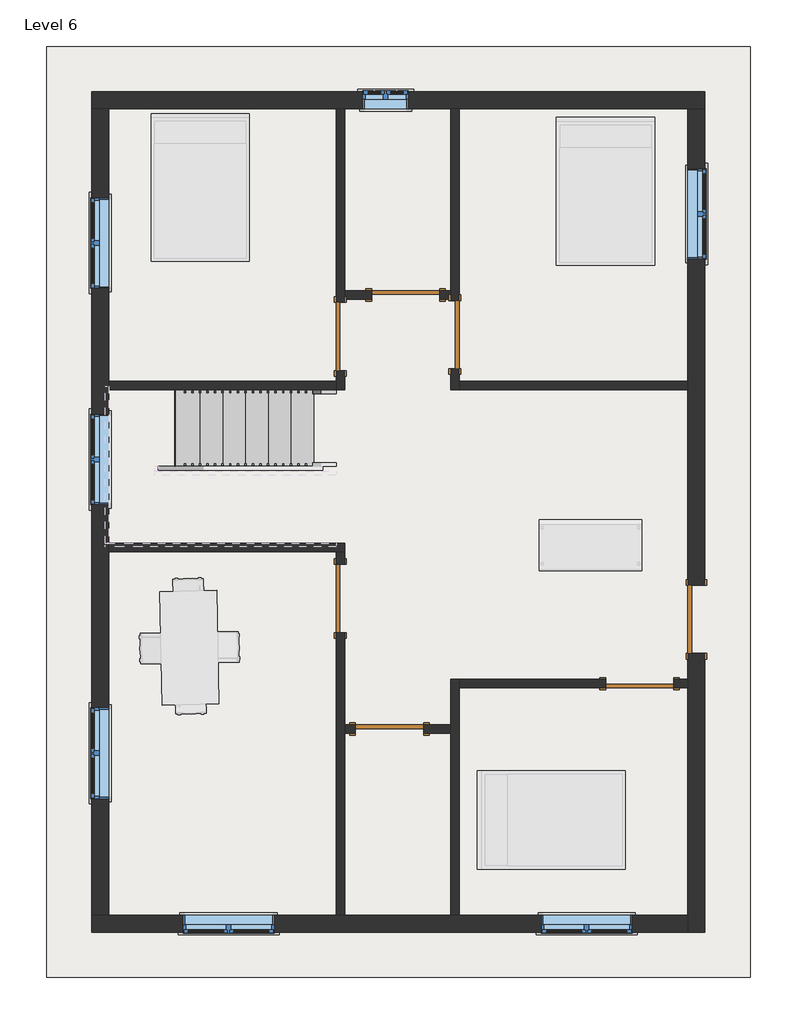
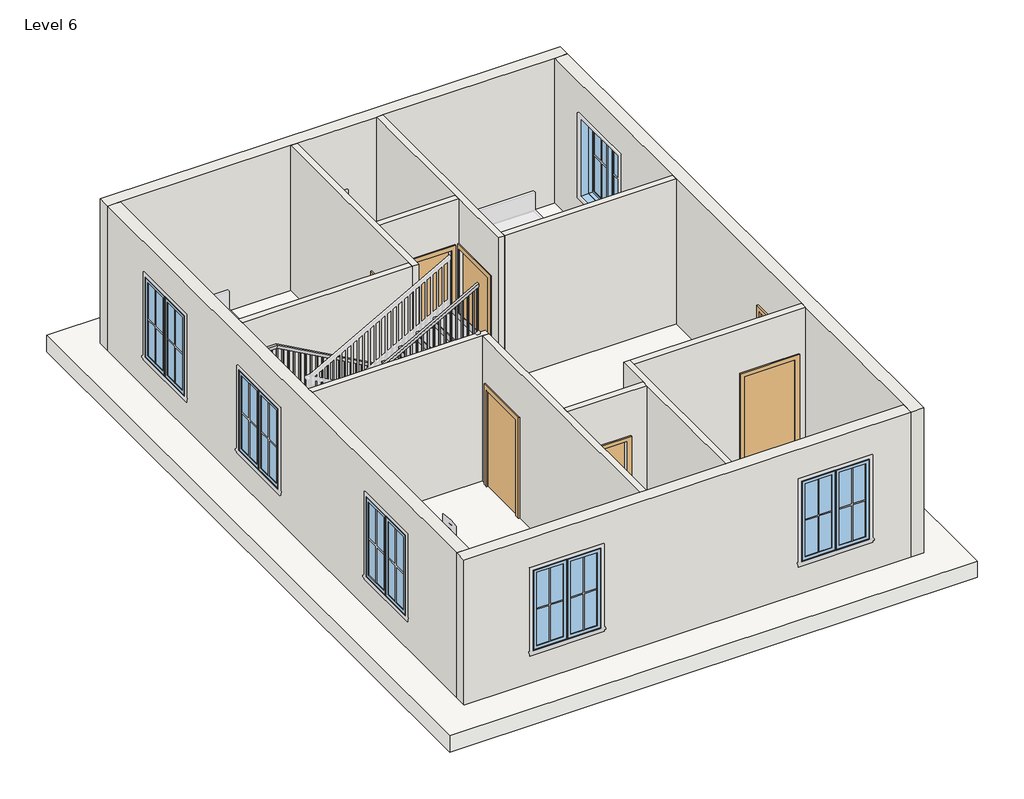
# One storey, part 1 of 2: 14 walls, 7 doors, 7 windows, 1 railing, 1 roof, 1 stair flight.
"""IFC4 building model written with IfcOpenShell, lengths in millimetres."""

from ifc_helpers import new_model, si_unit, frame, origin, place, context, project, spatial, polyline, outline, extrude, faceted_brep, transform, mapped, element, save
from components import door_e5f9f3c4, door_305aa2a5, door_a90ba1ad, stair_flight_597ccfed, window_c417fced, window_8377141f

model = new_model("IFC4")

# Units and contexts
model_context = context("Model", 3, world=origin())
ifc_project = project(units=[si_unit("LENGTHUNIT", "METRE", prefix="MILLI")], contexts=[model_context])

# Site, building, storey
site = spatial("IfcSite", under=ifc_project)
building = spatial("IfcBuilding", under=site)
storey = spatial("IfcBuildingStorey", under=building, Name="Level 6", Elevation=15240.0)

# Doors
placement = place(None, origin())
door_shape = door_e5f9f3c4(model_context)
element("IfcDoor", 1, ObjectType="Single-Flush : 36\" x 84\"", at=placement, inside=storey, context=model_context, shape_type="MappedRepresentation", body=[
    mapped(door_shape, transform((5226.05, 11245.85, 15240.0), x_axis=(1.0, 0.0, 0.0), y_axis=(0.0, 1.0, 0.0), z_axis=(0.0, 0.0, 1.0))),
])
element("IfcDoor", 2, ObjectType="Single-Flush : 36\" x 84\"", at=placement, inside=storey, context=model_context, shape_type="MappedRepresentation", body=[
    mapped(door_shape, transform((5886.45, 10712.45, 15240.0), x_axis=(0.0, -1.0, 0.0), y_axis=(1.0, 0.0, 0.0), z_axis=(0.0, 0.0, 1.0))),
])
door_2_shape = door_305aa2a5(model_context)
element("IfcDoor", 3, ObjectType="Single-Flush : 36\" x 84\"", at=placement, inside=storey, context=model_context, shape_type="MappedRepresentation", body=[
    mapped(door_2_shape, transform((4349.75, 10687.05, 15240.0), x_axis=(0.0, -1.0, 0.0), y_axis=(1.0, 0.0, 0.0), z_axis=(0.0, 0.0, 1.0))),
])
element("IfcDoor", 4, ObjectType="Single-Flush : 36\" x 84\"", at=placement, inside=storey, context=model_context, shape_type="MappedRepresentation", body=[
    mapped(door_2_shape, transform((8369.3, 6026.15, 15240.0), x_axis=(1.0, 0.0, 0.0), y_axis=(0.0, 1.0, 0.0), z_axis=(0.0, 0.0, 1.0))),
])
element("IfcDoor", 5, ObjectType="Single-Flush : 36\" x 84\"", at=placement, inside=storey, context=model_context, shape_type="MappedRepresentation", body=[
    mapped(door_2_shape, transform((5010.15, 5416.55, 15240.0), x_axis=(-1.0, 0.0, 0.0), y_axis=(0.0, -1.0, 0.0), z_axis=(0.0, 0.0, 1.0))),
])
element("IfcDoor", 6, ObjectType="Single-Flush : 36\" x 84\"", at=placement, inside=storey, context=model_context, shape_type="MappedRepresentation", body=[
    mapped(door_2_shape, transform((4349.75, 7169.15, 15240.0), x_axis=(0.0, -1.0, 0.0), y_axis=(1.0, 0.0, 0.0), z_axis=(0.0, 0.0, 1.0))),
])
door_3_shape = door_a90ba1ad(model_context)
element("IfcDoor", 7, ObjectType="Single-Flush : 36\" x 84\"", at=placement, inside=storey, context=model_context, shape_type="MappedRepresentation", body=[
    mapped(door_3_shape, transform((9131.3, 6889.75, 15240.0), x_axis=(0.0, -1.0, 0.0), y_axis=(1.0, 0.0, 0.0), z_axis=(0.0, 0.0, 1.0))),
])

# Railing
element("IfcRailing", 8, ObjectType="Handrail - Rectangular", at=placement, inside=storey, context=model_context, shape_type="SolidModel", body=[
    faceted_brep([(4295.1355783, 9918.7, 16323.7333333), (4295.1355783, 9918.7, 16265.620221), (4295.1355783, 9969.5, 16265.620221), (4295.1355783, 9969.5, 16323.7333333), (1856.7355783, 9918.7, 17678.4), (1843.5719761, 9918.7, 17627.6), (1843.5719761, 9969.5, 17627.6), (1856.7355783, 9969.5, 17678.4), (1295.4, 9918.7, 17678.4), (1295.4, 9918.7, 17627.6), (1244.6, 9969.5, 17627.6), (1244.6, 9969.5, 17678.4), (1295.4, 7962.9, 17678.4), (1295.4, 7962.9, 17627.6), (1244.6, 7912.1, 17627.6), (1244.6, 7912.1, 17678.4), (1551.9355783, 7962.9, 17678.4), (1565.0991806, 7962.9, 17627.6), (1565.0991806, 7912.1, 17627.6), (1551.9355783, 7912.1, 17678.4), (4295.1355783, 7962.9, 19202.4), (4295.1355783, 7912.1, 19202.4), (4295.1355783, 7912.1, 19144.2868876), (4295.1355783, 7962.9, 19144.2868876)], [[[0, 1, 2, 3]], [[1, 0, 4, 5]], [[2, 1, 5, 6]], [[3, 2, 6, 7]], [[0, 3, 7, 4]], [[5, 4, 8, 9]], [[6, 5, 9, 10]], [[7, 6, 10, 11]], [[4, 7, 11, 8]], [[9, 8, 12, 13]], [[10, 9, 13, 14]], [[11, 10, 14, 15]], [[8, 11, 15, 12]], [[13, 12, 16, 17]], [[14, 13, 17, 18]], [[15, 14, 18, 19]], [[12, 15, 19, 16]], [[20, 21, 22, 23]], [[17, 16, 20, 23]], [[18, 17, 23, 22]], [[19, 18, 22, 21]], [[16, 19, 21, 20]]]),
    extrude(outline(polyline([(19105.8365664, 4225.925), (19095.253233, 4206.875), (18118.6666667, 4206.875), (18118.6666667, 4225.925), (19105.8365664, 4225.925)])), frame((0.0, 7927.975, 0.0), z_axis=(0.0, 1.0, 0.0), x_axis=(0.0, 0.0, 1.0)), (0.0, 0.0, 1.0), 19.05),
    extrude(outline(polyline([(19049.3921219, 4124.325), (19038.8087886, 4105.275), (18118.6666667, 4105.275), (18118.6666667, 4124.325), (19049.3921219, 4124.325)])), frame((0.0, 7927.975, 0.0), z_axis=(0.0, 1.0, 0.0), x_axis=(0.0, 0.0, 1.0)), (0.0, 0.0, 1.0), 19.05),
    extrude(outline(polyline([(18992.9476775, 4022.725), (18982.3643441, 4003.675), (18118.6666667, 4003.675), (18118.6666667, 4022.725), (18992.9476775, 4022.725)])), frame((0.0, 7927.975, 0.0), z_axis=(0.0, 1.0, 0.0), x_axis=(0.0, 0.0, 1.0)), (0.0, 0.0, 1.0), 19.05),
    extrude(outline(polyline([(18936.503233, 3921.125), (18925.9198997, 3902.075), (17949.3333333, 3902.075), (17949.3333333, 3921.125), (18936.503233, 3921.125)])), frame((0.0, 7927.975, 0.0), z_axis=(0.0, 1.0, 0.0), x_axis=(0.0, 0.0, 1.0)), (0.0, 0.0, 1.0), 19.05),
    extrude(outline(polyline([(18880.0587886, 3819.525), (18869.4754552, 3800.475), (17949.3333333, 3800.475), (17949.3333333, 3819.525), (18880.0587886, 3819.525)])), frame((0.0, 7927.975, 0.0), z_axis=(0.0, 1.0, 0.0), x_axis=(0.0, 0.0, 1.0)), (0.0, 0.0, 1.0), 19.05),
    extrude(outline(polyline([(18823.6143441, 3717.925), (18813.0310108, 3698.875), (17949.3333333, 3698.875), (17949.3333333, 3717.925), (18823.6143441, 3717.925)])), frame((0.0, 7927.975, 0.0), z_axis=(0.0, 1.0, 0.0), x_axis=(0.0, 0.0, 1.0)), (0.0, 0.0, 1.0), 19.05),
    extrude(outline(polyline([(18767.1698997, 3616.325), (18756.5865664, 3597.275), (17780.0, 3597.275), (17780.0, 3616.325), (18767.1698997, 3616.325)])), frame((0.0, 7927.975, 0.0), z_axis=(0.0, 1.0, 0.0), x_axis=(0.0, 0.0, 1.0)), (0.0, 0.0, 1.0), 19.05),
    extrude(outline(polyline([(18710.7254552, 3514.725), (18700.1421219, 3495.675), (17780.0, 3495.675), (17780.0, 3514.725), (18710.7254552, 3514.725)])), frame((0.0, 7927.975, 0.0), z_axis=(0.0, 1.0, 0.0), x_axis=(0.0, 0.0, 1.0)), (0.0, 0.0, 1.0), 19.05),
    extrude(outline(polyline([(18654.2810108, 3413.125), (18643.6976775, 3394.075), (17780.0, 3394.075), (17780.0, 3413.125), (18654.2810108, 3413.125)])), frame((0.0, 7927.975, 0.0), z_axis=(0.0, 1.0, 0.0), x_axis=(0.0, 0.0, 1.0)), (0.0, 0.0, 1.0), 19.05),
    extrude(outline(polyline([(18597.8365664, 3311.525), (18587.253233, 3292.475), (17610.6666667, 3292.475), (17610.6666667, 3311.525), (18597.8365664, 3311.525)])), frame((0.0, 7927.975, 0.0), z_axis=(0.0, 1.0, 0.0), x_axis=(0.0, 0.0, 1.0)), (0.0, 0.0, 1.0), 19.05),
    extrude(outline(polyline([(18541.3921219, 3209.925), (18530.8087886, 3190.875), (17610.6666667, 3190.875), (17610.6666667, 3209.925), (18541.3921219, 3209.925)])), frame((0.0, 7927.975, 0.0), z_axis=(0.0, 1.0, 0.0), x_axis=(0.0, 0.0, 1.0)), (0.0, 0.0, 1.0), 19.05),
    extrude(outline(polyline([(18484.9476775, 3108.325), (18474.3643441, 3089.275), (17610.6666667, 3089.275), (17610.6666667, 3108.325), (18484.9476775, 3108.325)])), frame((0.0, 7927.975, 0.0), z_axis=(0.0, 1.0, 0.0), x_axis=(0.0, 0.0, 1.0)), (0.0, 0.0, 1.0), 19.05),
    extrude(outline(polyline([(18428.503233, 3006.725), (18417.9198997, 2987.675), (17441.3333333, 2987.675), (17441.3333333, 3006.725), (18428.503233, 3006.725)])), frame((0.0, 7927.975, 0.0), z_axis=(0.0, 1.0, 0.0), x_axis=(0.0, 0.0, 1.0)), (0.0, 0.0, 1.0), 19.05),
    extrude(outline(polyline([(18372.0587886, 2905.125), (18361.4754552, 2886.075), (17441.3333333, 2886.075), (17441.3333333, 2905.125), (18372.0587886, 2905.125)])), frame((0.0, 7927.975, 0.0), z_axis=(0.0, 1.0, 0.0), x_axis=(0.0, 0.0, 1.0)), (0.0, 0.0, 1.0), 19.05),
    extrude(outline(polyline([(18315.6143441, 2803.525), (18305.0310108, 2784.475), (17441.3333333, 2784.475), (17441.3333333, 2803.525), (18315.6143441, 2803.525)])), frame((0.0, 7927.975, 0.0), z_axis=(0.0, 1.0, 0.0), x_axis=(0.0, 0.0, 1.0)), (0.0, 0.0, 1.0), 19.05),
    extrude(outline(polyline([(18259.1698997, 2701.925), (18248.5865664, 2682.875), (17272.0, 2682.875), (17272.0, 2701.925), (18259.1698997, 2701.925)])), frame((0.0, 7927.975, 0.0), z_axis=(0.0, 1.0, 0.0), x_axis=(0.0, 0.0, 1.0)), (0.0, 0.0, 1.0), 19.05),
    extrude(outline(polyline([(18202.7254552, 2600.325), (18192.1421219, 2581.275), (17272.0, 2581.275), (17272.0, 2600.325), (18202.7254552, 2600.325)])), frame((0.0, 7927.975, 0.0), z_axis=(0.0, 1.0, 0.0), x_axis=(0.0, 0.0, 1.0)), (0.0, 0.0, 1.0), 19.05),
    extrude(outline(polyline([(18146.2810108, 2498.725), (18135.6976775, 2479.675), (17272.0, 2479.675), (17272.0, 2498.725), (18146.2810108, 2498.725)])), frame((0.0, 7927.975, 0.0), z_axis=(0.0, 1.0, 0.0), x_axis=(0.0, 0.0, 1.0)), (0.0, 0.0, 1.0), 19.05),
    extrude(outline(polyline([(18089.8365664, 2397.125), (18079.253233, 2378.075), (17102.6666667, 2378.075), (17102.6666667, 2397.125), (18089.8365664, 2397.125)])), frame((0.0, 7927.975, 0.0), z_axis=(0.0, 1.0, 0.0), x_axis=(0.0, 0.0, 1.0)), (0.0, 0.0, 1.0), 19.05),
    extrude(outline(polyline([(18033.3921219, 2295.525), (18022.8087886, 2276.475), (17102.6666667, 2276.475), (17102.6666667, 2295.525), (18033.3921219, 2295.525)])), frame((0.0, 7927.975, 0.0), z_axis=(0.0, 1.0, 0.0), x_axis=(0.0, 0.0, 1.0)), (0.0, 0.0, 1.0), 19.05),
    extrude(outline(polyline([(17976.9476775, 2193.925), (17966.3643441, 2174.875), (17102.6666667, 2174.875), (17102.6666667, 2193.925), (17976.9476775, 2193.925)])), frame((0.0, 7927.975, 0.0), z_axis=(0.0, 1.0, 0.0), x_axis=(0.0, 0.0, 1.0)), (0.0, 0.0, 1.0), 19.05),
    extrude(outline(polyline([(17920.503233, 2092.325), (17909.9198997, 2073.275), (16933.3333333, 2073.275), (16933.3333333, 2092.325), (17920.503233, 2092.325)])), frame((0.0, 7927.975, 0.0), z_axis=(0.0, 1.0, 0.0), x_axis=(0.0, 0.0, 1.0)), (0.0, 0.0, 1.0), 19.05),
    extrude(outline(polyline([(17864.0587886, 1990.725), (17853.4754552, 1971.675), (16933.3333333, 1971.675), (16933.3333333, 1990.725), (17864.0587886, 1990.725)])), frame((0.0, 7927.975, 0.0), z_axis=(0.0, 1.0, 0.0), x_axis=(0.0, 0.0, 1.0)), (0.0, 0.0, 1.0), 19.05),
    extrude(outline(polyline([(17807.6143441, 1889.125), (17797.0310108, 1870.075), (16933.3333333, 1870.075), (16933.3333333, 1889.125), (17807.6143441, 1889.125)])), frame((0.0, 7927.975, 0.0), z_axis=(0.0, 1.0, 0.0), x_axis=(0.0, 0.0, 1.0)), (0.0, 0.0, 1.0), 19.05),
    extrude(outline(polyline([(17751.1698997, 1787.525), (17740.5865664, 1768.475), (16764.0, 1768.475), (16764.0, 1787.525), (17751.1698997, 1787.525)])), frame((0.0, 7927.975, 0.0), z_axis=(0.0, 1.0, 0.0), x_axis=(0.0, 0.0, 1.0)), (0.0, 0.0, 1.0), 19.05),
    extrude(outline(polyline([(17694.7254552, 1685.925), (17684.1421219, 1666.875), (16764.0, 1666.875), (16764.0, 1685.925), (17694.7254552, 1685.925)])), frame((0.0, 7927.975, 0.0), z_axis=(0.0, 1.0, 0.0), x_axis=(0.0, 0.0, 1.0)), (0.0, 0.0, 1.0), 19.05),
    extrude(outline(polyline([(17638.2810108, 1584.325), (17627.6976775, 1565.275), (16764.0, 1565.275), (16764.0, 1584.325), (17638.2810108, 1584.325)])), frame((0.0, 7927.975, 0.0), z_axis=(0.0, 1.0, 0.0), x_axis=(0.0, 0.0, 1.0)), (0.0, 0.0, 1.0), 19.05),
    extrude(outline(polyline([(1463.675, 7927.975), (1463.675, 7947.025), (1482.725, 7947.025), (1482.725, 7927.975), (1463.675, 7927.975)])), frame((0.0, 0.0, 16764.0), z_axis=(0.0, 0.0, 1.0), x_axis=(1.0, 0.0, 0.0)), (0.0, 0.0, 1.0), 863.6),
    extrude(outline(polyline([(1362.075, 7927.975), (1362.075, 7947.025), (1381.125, 7947.025), (1381.125, 7927.975), (1362.075, 7927.975)])), frame((0.0, 0.0, 16764.0), z_axis=(0.0, 0.0, 1.0), x_axis=(1.0, 0.0, 0.0)), (0.0, 0.0, 1.0), 863.6),
    extrude(outline(polyline([(1260.475, 8023.225), (1279.525, 8023.225), (1279.525, 8004.175), (1260.475, 8004.175), (1260.475, 8023.225)])), frame((0.0, 0.0, 16764.0), z_axis=(0.0, 0.0, 1.0), x_axis=(1.0, 0.0, 0.0)), (0.0, 0.0, 1.0), 863.6),
    extrude(outline(polyline([(1260.475, 8124.825), (1279.525, 8124.825), (1279.525, 8105.775), (1260.475, 8105.775), (1260.475, 8124.825)])), frame((0.0, 0.0, 16764.0), z_axis=(0.0, 0.0, 1.0), x_axis=(1.0, 0.0, 0.0)), (0.0, 0.0, 1.0), 863.6),
    extrude(outline(polyline([(1260.475, 8226.425), (1279.525, 8226.425), (1279.525, 8207.375), (1260.475, 8207.375), (1260.475, 8226.425)])), frame((0.0, 0.0, 16764.0), z_axis=(0.0, 0.0, 1.0), x_axis=(1.0, 0.0, 0.0)), (0.0, 0.0, 1.0), 863.6),
    extrude(outline(polyline([(1260.475, 8328.025), (1279.525, 8328.025), (1279.525, 8308.975), (1260.475, 8308.975), (1260.475, 8328.025)])), frame((0.0, 0.0, 16764.0), z_axis=(0.0, 0.0, 1.0), x_axis=(1.0, 0.0, 0.0)), (0.0, 0.0, 1.0), 863.6),
    extrude(outline(polyline([(1260.475, 8429.625), (1279.525, 8429.625), (1279.525, 8410.575), (1260.475, 8410.575), (1260.475, 8429.625)])), frame((0.0, 0.0, 16764.0), z_axis=(0.0, 0.0, 1.0), x_axis=(1.0, 0.0, 0.0)), (0.0, 0.0, 1.0), 863.6),
    extrude(outline(polyline([(1260.475, 8531.225), (1279.525, 8531.225), (1279.525, 8512.175), (1260.475, 8512.175), (1260.475, 8531.225)])), frame((0.0, 0.0, 16764.0), z_axis=(0.0, 0.0, 1.0), x_axis=(1.0, 0.0, 0.0)), (0.0, 0.0, 1.0), 863.6),
    extrude(outline(polyline([(1260.475, 8632.825), (1279.525, 8632.825), (1279.525, 8613.775), (1260.475, 8613.775), (1260.475, 8632.825)])), frame((0.0, 0.0, 16764.0), z_axis=(0.0, 0.0, 1.0), x_axis=(1.0, 0.0, 0.0)), (0.0, 0.0, 1.0), 863.6),
    extrude(outline(polyline([(1260.475, 8734.425), (1279.525, 8734.425), (1279.525, 8715.375), (1260.475, 8715.375), (1260.475, 8734.425)])), frame((0.0, 0.0, 16764.0), z_axis=(0.0, 0.0, 1.0), x_axis=(1.0, 0.0, 0.0)), (0.0, 0.0, 1.0), 863.6),
    extrude(outline(polyline([(1260.475, 8836.025), (1279.525, 8836.025), (1279.525, 8816.975), (1260.475, 8816.975), (1260.475, 8836.025)])), frame((0.0, 0.0, 16764.0), z_axis=(0.0, 0.0, 1.0), x_axis=(1.0, 0.0, 0.0)), (0.0, 0.0, 1.0), 863.6),
    extrude(outline(polyline([(1260.475, 8937.625), (1279.525, 8937.625), (1279.525, 8918.575), (1260.475, 8918.575), (1260.475, 8937.625)])), frame((0.0, 0.0, 16764.0), z_axis=(0.0, 0.0, 1.0), x_axis=(1.0, 0.0, 0.0)), (0.0, 0.0, 1.0), 863.6),
    extrude(outline(polyline([(1260.475, 9039.225), (1279.525, 9039.225), (1279.525, 9020.175), (1260.475, 9020.175), (1260.475, 9039.225)])), frame((0.0, 0.0, 16764.0), z_axis=(0.0, 0.0, 1.0), x_axis=(1.0, 0.0, 0.0)), (0.0, 0.0, 1.0), 863.6),
    extrude(outline(polyline([(1260.475, 9140.825), (1279.525, 9140.825), (1279.525, 9121.775), (1260.475, 9121.775), (1260.475, 9140.825)])), frame((0.0, 0.0, 16764.0), z_axis=(0.0, 0.0, 1.0), x_axis=(1.0, 0.0, 0.0)), (0.0, 0.0, 1.0), 863.6),
    extrude(outline(polyline([(1260.475, 9242.425), (1279.525, 9242.425), (1279.525, 9223.375), (1260.475, 9223.375), (1260.475, 9242.425)])), frame((0.0, 0.0, 16764.0), z_axis=(0.0, 0.0, 1.0), x_axis=(1.0, 0.0, 0.0)), (0.0, 0.0, 1.0), 863.6),
    extrude(outline(polyline([(1260.475, 9344.025), (1279.525, 9344.025), (1279.525, 9324.975), (1260.475, 9324.975), (1260.475, 9344.025)])), frame((0.0, 0.0, 16764.0), z_axis=(0.0, 0.0, 1.0), x_axis=(1.0, 0.0, 0.0)), (0.0, 0.0, 1.0), 863.6),
    extrude(outline(polyline([(1260.475, 9445.625), (1279.525, 9445.625), (1279.525, 9426.575), (1260.475, 9426.575), (1260.475, 9445.625)])), frame((0.0, 0.0, 16764.0), z_axis=(0.0, 0.0, 1.0), x_axis=(1.0, 0.0, 0.0)), (0.0, 0.0, 1.0), 863.6),
    extrude(outline(polyline([(1260.475, 9547.225), (1279.525, 9547.225), (1279.525, 9528.175), (1260.475, 9528.175), (1260.475, 9547.225)])), frame((0.0, 0.0, 16764.0), z_axis=(0.0, 0.0, 1.0), x_axis=(1.0, 0.0, 0.0)), (0.0, 0.0, 1.0), 863.6),
    extrude(outline(polyline([(1260.475, 9648.825), (1279.525, 9648.825), (1279.525, 9629.775), (1260.475, 9629.775), (1260.475, 9648.825)])), frame((0.0, 0.0, 16764.0), z_axis=(0.0, 0.0, 1.0), x_axis=(1.0, 0.0, 0.0)), (0.0, 0.0, 1.0), 863.6),
    extrude(outline(polyline([(1260.475, 9750.425), (1279.525, 9750.425), (1279.525, 9731.375), (1260.475, 9731.375), (1260.475, 9750.425)])), frame((0.0, 0.0, 16764.0), z_axis=(0.0, 0.0, 1.0), x_axis=(1.0, 0.0, 0.0)), (0.0, 0.0, 1.0), 863.6),
    extrude(outline(polyline([(1260.475, 9852.025), (1279.525, 9852.025), (1279.525, 9832.975), (1260.475, 9832.975), (1260.475, 9852.025)])), frame((0.0, 0.0, 16764.0), z_axis=(0.0, 0.0, 1.0), x_axis=(1.0, 0.0, 0.0)), (0.0, 0.0, 1.0), 863.6),
    extrude(outline(polyline([(1358.2605783, 9953.625), (1358.2605783, 9934.575), (1339.2105783, 9934.575), (1339.2105783, 9953.625), (1358.2605783, 9953.625)])), frame((0.0, 0.0, 16764.0), z_axis=(0.0, 0.0, 1.0), x_axis=(1.0, 0.0, 0.0)), (0.0, 0.0, 1.0), 863.6),
    extrude(outline(polyline([(1459.8605783, 9953.625), (1459.8605783, 9934.575), (1440.8105783, 9934.575), (1440.8105783, 9953.625), (1459.8605783, 9953.625)])), frame((0.0, 0.0, 16764.0), z_axis=(0.0, 0.0, 1.0), x_axis=(1.0, 0.0, 0.0)), (0.0, 0.0, 1.0), 863.6),
    extrude(outline(polyline([(1561.4605783, 9953.625), (1561.4605783, 9934.575), (1542.4105783, 9934.575), (1542.4105783, 9953.625), (1561.4605783, 9953.625)])), frame((0.0, 0.0, 16764.0), z_axis=(0.0, 0.0, 1.0), x_axis=(1.0, 0.0, 0.0)), (0.0, 0.0, 1.0), 863.6),
    extrude(outline(polyline([(1663.0605783, 9953.625), (1663.0605783, 9934.575), (1644.0105783, 9934.575), (1644.0105783, 9953.625), (1663.0605783, 9953.625)])), frame((0.0, 0.0, 16764.0), z_axis=(0.0, 0.0, 1.0), x_axis=(1.0, 0.0, 0.0)), (0.0, 0.0, 1.0), 863.6),
    extrude(outline(polyline([(1764.6605783, 9953.625), (1764.6605783, 9934.575), (1745.6105783, 9934.575), (1745.6105783, 9953.625), (1764.6605783, 9953.625)])), frame((0.0, 0.0, 16764.0), z_axis=(0.0, 0.0, 1.0), x_axis=(1.0, 0.0, 0.0)), (0.0, 0.0, 1.0), 863.6),
    extrude(outline(polyline([(17614.995221, 1866.2605783), (17625.5785543, 1847.2105783), (16764.0, 1847.2105783), (16764.0, 1866.2605783), (17614.995221, 1866.2605783)])), frame((0.0, 9934.575, 0.0), z_axis=(0.0, 1.0, 0.0), x_axis=(0.0, 0.0, 1.0)), (0.0, 0.0, 1.0), 19.05),
    extrude(outline(polyline([(17558.5507765, 1967.8605783), (17569.1341099, 1948.8105783), (16594.6666667, 1948.8105783), (16594.6666667, 1967.8605783), (17558.5507765, 1967.8605783)])), frame((0.0, 9934.575, 0.0), z_axis=(0.0, 1.0, 0.0), x_axis=(0.0, 0.0, 1.0)), (0.0, 0.0, 1.0), 19.05),
    extrude(outline(polyline([(17502.1063321, 2069.4605783), (17512.6896654, 2050.4105783), (16594.6666667, 2050.4105783), (16594.6666667, 2069.4605783), (17502.1063321, 2069.4605783)])), frame((0.0, 9934.575, 0.0), z_axis=(0.0, 1.0, 0.0), x_axis=(0.0, 0.0, 1.0)), (0.0, 0.0, 1.0), 19.05),
    extrude(outline(polyline([(17445.6618876, 2171.0605783), (17456.245221, 2152.0105783), (16594.6666667, 2152.0105783), (16594.6666667, 2171.0605783), (17445.6618876, 2171.0605783)])), frame((0.0, 9934.575, 0.0), z_axis=(0.0, 1.0, 0.0), x_axis=(0.0, 0.0, 1.0)), (0.0, 0.0, 1.0), 19.05),
    extrude(outline(polyline([(17389.2174432, 2272.6605783), (17399.8007765, 2253.6105783), (16425.3333333, 2253.6105783), (16425.3333333, 2272.6605783), (17389.2174432, 2272.6605783)])), frame((0.0, 9934.575, 0.0), z_axis=(0.0, 1.0, 0.0), x_axis=(0.0, 0.0, 1.0)), (0.0, 0.0, 1.0), 19.05),
    extrude(outline(polyline([(17332.7729988, 2374.2605783), (17343.3563321, 2355.2105783), (16425.3333333, 2355.2105783), (16425.3333333, 2374.2605783), (17332.7729988, 2374.2605783)])), frame((0.0, 9934.575, 0.0), z_axis=(0.0, 1.0, 0.0), x_axis=(0.0, 0.0, 1.0)), (0.0, 0.0, 1.0), 19.05),
    extrude(outline(polyline([(17276.3285543, 2475.8605783), (17286.9118876, 2456.8105783), (16425.3333333, 2456.8105783), (16425.3333333, 2475.8605783), (17276.3285543, 2475.8605783)])), frame((0.0, 9934.575, 0.0), z_axis=(0.0, 1.0, 0.0), x_axis=(0.0, 0.0, 1.0)), (0.0, 0.0, 1.0), 19.05),
    extrude(outline(polyline([(17219.8841099, 2577.4605783), (17230.4674432, 2558.4105783), (16256.0, 2558.4105783), (16256.0, 2577.4605783), (17219.8841099, 2577.4605783)])), frame((0.0, 9934.575, 0.0), z_axis=(0.0, 1.0, 0.0), x_axis=(0.0, 0.0, 1.0)), (0.0, 0.0, 1.0), 19.05),
    extrude(outline(polyline([(17163.4396654, 2679.0605783), (17174.0229988, 2660.0105783), (16256.0, 2660.0105783), (16256.0, 2679.0605783), (17163.4396654, 2679.0605783)])), frame((0.0, 9934.575, 0.0), z_axis=(0.0, 1.0, 0.0), x_axis=(0.0, 0.0, 1.0)), (0.0, 0.0, 1.0), 19.05),
    extrude(outline(polyline([(17106.995221, 2780.6605783), (17117.5785543, 2761.6105783), (16256.0, 2761.6105783), (16256.0, 2780.6605783), (17106.995221, 2780.6605783)])), frame((0.0, 9934.575, 0.0), z_axis=(0.0, 1.0, 0.0), x_axis=(0.0, 0.0, 1.0)), (0.0, 0.0, 1.0), 19.05),
    extrude(outline(polyline([(17050.5507765, 2882.2605783), (17061.1341099, 2863.2105783), (16086.6666667, 2863.2105783), (16086.6666667, 2882.2605783), (17050.5507765, 2882.2605783)])), frame((0.0, 9934.575, 0.0), z_axis=(0.0, 1.0, 0.0), x_axis=(0.0, 0.0, 1.0)), (0.0, 0.0, 1.0), 19.05),
    extrude(outline(polyline([(16994.1063321, 2983.8605783), (17004.6896654, 2964.8105783), (16086.6666667, 2964.8105783), (16086.6666667, 2983.8605783), (16994.1063321, 2983.8605783)])), frame((0.0, 9934.575, 0.0), z_axis=(0.0, 1.0, 0.0), x_axis=(0.0, 0.0, 1.0)), (0.0, 0.0, 1.0), 19.05),
    extrude(outline(polyline([(16937.6618876, 3085.4605783), (16948.245221, 3066.4105783), (16086.6666667, 3066.4105783), (16086.6666667, 3085.4605783), (16937.6618876, 3085.4605783)])), frame((0.0, 9934.575, 0.0), z_axis=(0.0, 1.0, 0.0), x_axis=(0.0, 0.0, 1.0)), (0.0, 0.0, 1.0), 19.05),
    extrude(outline(polyline([(16881.2174432, 3187.0605783), (16891.8007765, 3168.0105783), (15917.3333333, 3168.0105783), (15917.3333333, 3187.0605783), (16881.2174432, 3187.0605783)])), frame((0.0, 9934.575, 0.0), z_axis=(0.0, 1.0, 0.0), x_axis=(0.0, 0.0, 1.0)), (0.0, 0.0, 1.0), 19.05),
    extrude(outline(polyline([(16824.7729988, 3288.6605783), (16835.3563321, 3269.6105783), (15917.3333333, 3269.6105783), (15917.3333333, 3288.6605783), (16824.7729988, 3288.6605783)])), frame((0.0, 9934.575, 0.0), z_axis=(0.0, 1.0, 0.0), x_axis=(0.0, 0.0, 1.0)), (0.0, 0.0, 1.0), 19.05),
    extrude(outline(polyline([(16768.3285543, 3390.2605783), (16778.9118876, 3371.2105783), (15917.3333333, 3371.2105783), (15917.3333333, 3390.2605783), (16768.3285543, 3390.2605783)])), frame((0.0, 9934.575, 0.0), z_axis=(0.0, 1.0, 0.0), x_axis=(0.0, 0.0, 1.0)), (0.0, 0.0, 1.0), 19.05),
    extrude(outline(polyline([(16711.8841099, 3491.8605783), (16722.4674432, 3472.8105783), (15748.0, 3472.8105783), (15748.0, 3491.8605783), (16711.8841099, 3491.8605783)])), frame((0.0, 9934.575, 0.0), z_axis=(0.0, 1.0, 0.0), x_axis=(0.0, 0.0, 1.0)), (0.0, 0.0, 1.0), 19.05),
    extrude(outline(polyline([(16655.4396654, 3593.4605783), (16666.0229988, 3574.4105783), (15748.0, 3574.4105783), (15748.0, 3593.4605783), (16655.4396654, 3593.4605783)])), frame((0.0, 9934.575, 0.0), z_axis=(0.0, 1.0, 0.0), x_axis=(0.0, 0.0, 1.0)), (0.0, 0.0, 1.0), 19.05),
    extrude(outline(polyline([(16598.995221, 3695.0605783), (16609.5785543, 3676.0105783), (15748.0, 3676.0105783), (15748.0, 3695.0605783), (16598.995221, 3695.0605783)])), frame((0.0, 9934.575, 0.0), z_axis=(0.0, 1.0, 0.0), x_axis=(0.0, 0.0, 1.0)), (0.0, 0.0, 1.0), 19.05),
    extrude(outline(polyline([(16542.5507765, 3796.6605783), (16553.1341099, 3777.6105783), (15578.6666667, 3777.6105783), (15578.6666667, 3796.6605783), (16542.5507765, 3796.6605783)])), frame((0.0, 9934.575, 0.0), z_axis=(0.0, 1.0, 0.0), x_axis=(0.0, 0.0, 1.0)), (0.0, 0.0, 1.0), 19.05),
    extrude(outline(polyline([(16486.1063321, 3898.2605783), (16496.6896654, 3879.2105783), (15578.6666667, 3879.2105783), (15578.6666667, 3898.2605783), (16486.1063321, 3898.2605783)])), frame((0.0, 9934.575, 0.0), z_axis=(0.0, 1.0, 0.0), x_axis=(0.0, 0.0, 1.0)), (0.0, 0.0, 1.0), 19.05),
    extrude(outline(polyline([(16429.6618876, 3999.8605783), (16440.245221, 3980.8105783), (15578.6666667, 3980.8105783), (15578.6666667, 3999.8605783), (16429.6618876, 3999.8605783)])), frame((0.0, 9934.575, 0.0), z_axis=(0.0, 1.0, 0.0), x_axis=(0.0, 0.0, 1.0)), (0.0, 0.0, 1.0), 19.05),
    extrude(outline(polyline([(16373.2174432, 4101.4605783), (16383.8007765, 4082.4105783), (15409.3333333, 4082.4105783), (15409.3333333, 4101.4605783), (16373.2174432, 4101.4605783)])), frame((0.0, 9934.575, 0.0), z_axis=(0.0, 1.0, 0.0), x_axis=(0.0, 0.0, 1.0)), (0.0, 0.0, 1.0), 19.05),
    extrude(outline(polyline([(16316.7729988, 4203.0605783), (16327.3563321, 4184.0105783), (15409.3333333, 4184.0105783), (15409.3333333, 4203.0605783), (16316.7729988, 4203.0605783)])), frame((0.0, 9934.575, 0.0), z_axis=(0.0, 1.0, 0.0), x_axis=(0.0, 0.0, 1.0)), (0.0, 0.0, 1.0), 19.05),
    extrude(outline(polyline([(1260.475, 7947.025), (1279.525, 7947.025), (1279.525, 7927.975), (1260.475, 7927.975), (1260.475, 7947.025)])), frame((0.0, 0.0, 16764.0), z_axis=(0.0, 0.0, 1.0), x_axis=(1.0, 0.0, 0.0)), (0.0, 0.0, 1.0), 863.6),
    extrude(outline(polyline([(1279.525, 9953.625), (1279.525, 9934.575), (1260.475, 9934.575), (1260.475, 9953.625), (1279.525, 9953.625)])), frame((0.0, 0.0, 16764.0), z_axis=(0.0, 0.0, 1.0), x_axis=(1.0, 0.0, 0.0)), (0.0, 0.0, 1.0), 863.6),
    extrude(outline(polyline([(19144.2868876, 4295.1355783), (19133.7035543, 4276.0855783), (18118.6666667, 4276.0855783), (18118.6666667, 4295.1355783), (19144.2868876, 4295.1355783)])), frame((0.0, 7927.975, 0.0), z_axis=(0.0, 1.0, 0.0), x_axis=(0.0, 0.0, 1.0)), (0.0, 0.0, 1.0), 19.05),
    extrude(outline(polyline([(16265.620221, 4295.1355783), (16276.2035543, 4276.0855783), (15409.3333333, 4276.0855783), (15409.3333333, 4295.1355783), (16265.620221, 4295.1355783)])), frame((0.0, 9934.575, 0.0), z_axis=(0.0, 1.0, 0.0), x_axis=(0.0, 0.0, 1.0)), (0.0, 0.0, 1.0), 19.05),
])

# Roof
element("IfcRoof", 9, ObjectType="Generic - 12\"", at=placement, inside=storey, context=model_context, shape_type="SweptSolid", body=[
    extrude(outline(polyline([(406.4, 14579.6), (9855.2, 14579.6), (9855.2, 2082.8), (406.4, 2082.8), (406.4, 14579.6)])), frame((0.0, 0.0, 15240.0), z_axis=(0.0, 0.0, 1.0), x_axis=(1.0, 0.0, 0.0)), (0.0, 0.0, 1.0), 304.8),
])

# Stair flight
stair_flight_shape = stair_flight_597ccfed(model_context)
element("IfcStairFlight", 10, ObjectType="2\" Tread 1\" Nosing 1/4\" Riser", at=placement, inside=storey, context=model_context, shape_type="MappedRepresentation", body=[
    mapped(stair_flight_shape, transform((0.0, 0.0, 0.0), x_axis=(1.0, 0.0, 0.0), y_axis=(0.0, 1.0, 0.0), z_axis=(0.0, 0.0, 1.0))),
])

# Walls
element("IfcWall", 11, ObjectType="Generic - 5\"", at=placement, inside=storey, context=model_context, shape_type="Brep", body=[
    faceted_brep([(4292.6, 10229.85, 17373.6), (4292.6, 10229.85, 15240.0), (4292.6, 10083.8, 15240.0), (4292.6, 9969.5, 15240.0), (4292.6, 9969.5, 18288.0), (4292.6, 10083.8, 18288.0), (4292.6, 13741.4, 18288.0), (4292.6, 13741.4, 15240.0), (4292.6, 11144.25, 15240.0), (4292.6, 11144.25, 17373.6), (4406.9, 9969.5, 15240.0), (4406.9, 10229.85, 15240.0), (4406.9, 10229.85, 17373.6), (4406.9, 11144.25, 17373.6), (4406.9, 11144.25, 15240.0), (4406.9, 11188.7, 15240.0), (4406.9, 11303.0, 15240.0), (4406.9, 13741.4, 15240.0), (4406.9, 13741.4, 18288.0), (4406.9, 11303.0, 18288.0), (4406.9, 11188.7, 18288.0), (4406.9, 9969.5, 18288.0)], [[[0, 1, 2, 3, 4, 5, 6, 7, 8, 9]], [[10, 11, 12, 13, 14, 15, 16, 17, 18, 19, 20, 21]], [[8, 7, 17, 16, 15, 14]], [[3, 2, 1, 11, 10]], [[6, 5, 4, 21, 20, 19, 18]], [[7, 6, 18, 17]], [[4, 3, 10, 21]], [[12, 11, 1, 0]], [[13, 12, 0, 9]], [[14, 13, 9, 8]]]),
])
element("IfcWall", 12, ObjectType="Generic - 5\"", at=placement, inside=storey, context=model_context, shape_type="SweptSolid", body=[
    extrude(outline(polyline([(1244.6, 10083.8), (4292.6, 10083.8), (4292.6, 9969.5), (1244.6, 9969.5), (1244.6, 10083.8)])), frame((0.0, 0.0, 15240.0), z_axis=(0.0, 0.0, 1.0), x_axis=(1.0, 0.0, 0.0)), (0.0, 0.0, 1.0), 3048.0),
])
element("IfcWall", 13, ObjectType="Generic - 5\"", at=placement, inside=storey, context=model_context, shape_type="SweptSolid", body=[
    extrude(outline(polyline([(17373.6, 5683.25), (15240.0, 5683.25), (15240.0, 5829.3), (18288.0, 5829.3), (18288.0, 4406.9), (15240.0, 4406.9), (15240.0, 4768.85), (17373.6, 4768.85), (17373.6, 5683.25)])), frame((0.0, 11188.7, 0.0), z_axis=(0.0, 1.0, 0.0), x_axis=(0.0, 0.0, 1.0)), (0.0, 0.0, 1.0), 114.3),
])
element("IfcWall", 14, ObjectType="Generic - 5\"", at=placement, inside=storey, context=model_context, shape_type="Brep", body=[
    faceted_brep([(5829.3, 10255.25, 17373.6), (5829.3, 10255.25, 15240.0), (5829.3, 9969.5, 15240.0), (5829.3, 9969.5, 18288.0), (5829.3, 11188.7, 18288.0), (5829.3, 11303.0, 18288.0), (5829.3, 13741.4, 18288.0), (5829.3, 13741.4, 15240.0), (5829.3, 11303.0, 15240.0), (5829.3, 11188.7, 15240.0), (5829.3, 11169.65, 15240.0), (5829.3, 11169.65, 17373.6), (5943.6, 9969.5, 15240.0), (5943.6, 10083.8, 15240.0), (5943.6, 10255.25, 15240.0), (5943.6, 10255.25, 17373.6), (5943.6, 11169.65, 17373.6), (5943.6, 11169.65, 15240.0), (5943.6, 13741.4, 15240.0), (5943.6, 13741.4, 18288.0), (5943.6, 10083.8, 18288.0), (5943.6, 9969.5, 18288.0)], [[[0, 1, 2, 3, 4, 5, 6, 7, 8, 9, 10, 11]], [[12, 13, 14, 15, 16, 17, 18, 19, 20, 21]], [[2, 1, 14, 13, 12]], [[10, 9, 8, 7, 18, 17]], [[6, 5, 4, 3, 21, 20, 19]], [[7, 6, 19, 18]], [[3, 2, 12, 21]], [[15, 14, 1, 0]], [[16, 15, 0, 11]], [[17, 16, 11, 10]]]),
])
element("IfcWall", 15, ObjectType="Generic - 5\"", at=placement, inside=storey, context=model_context, shape_type="SweptSolid", body=[
    extrude(outline(polyline([(9017.0, 9969.5), (5943.6, 9969.5), (5943.6, 10083.8), (9017.0, 10083.8), (9017.0, 9969.5)])), frame((0.0, 0.0, 15240.0), z_axis=(0.0, 0.0, 1.0), x_axis=(1.0, 0.0, 0.0)), (0.0, 0.0, 1.0), 3048.0),
])
element("IfcWall", 16, ObjectType="Generic - 5\"", at=placement, inside=storey, context=model_context, shape_type="Brep", body=[
    faceted_brep([(1244.6, 7797.8, 15240.0), (4292.6, 7797.8, 15240.0), (4406.9, 7797.8, 15240.0), (4406.9, 7797.8, 18288.0), (4292.6, 7797.8, 18288.0), (1244.6, 7797.8, 18288.0), (1244.6, 7912.1, 15240.0), (1244.6, 7912.1, 18288.0), (4406.9, 7912.1, 18288.0), (4406.9, 7912.1, 15240.0)], [[[0, 1, 2, 3, 4, 5]], [[6, 7, 8, 9]], [[2, 1, 0, 6, 9]], [[5, 4, 3, 8, 7]], [[0, 5, 7, 6]], [[3, 2, 9, 8]]]),
])
element("IfcWall", 17, ObjectType="Generic - 5\"", at=placement, inside=storey, context=model_context, shape_type="Brep", body=[
    faceted_brep([(4292.6, 6711.95, 17373.6), (4292.6, 6711.95, 15240.0), (4292.6, 2921.0, 15240.0), (4292.6, 2921.0, 18288.0), (4292.6, 7797.8, 18288.0), (4292.6, 7797.8, 15240.0), (4292.6, 7626.35, 15240.0), (4292.6, 7626.35, 17373.6), (4406.9, 2921.0, 15240.0), (4406.9, 5359.4, 15240.0), (4406.9, 5473.7, 15240.0), (4406.9, 6711.95, 15240.0), (4406.9, 6711.95, 17373.6), (4406.9, 7626.35, 17373.6), (4406.9, 7626.35, 15240.0), (4406.9, 7797.8, 15240.0), (4406.9, 7797.8, 18288.0), (4406.9, 5473.7, 18288.0), (4406.9, 5359.4, 18288.0), (4406.9, 2921.0, 18288.0)], [[[0, 1, 2, 3, 4, 5, 6, 7]], [[8, 9, 10, 11, 12, 13, 14, 15, 16, 17, 18, 19]], [[6, 5, 15, 14]], [[2, 1, 11, 10, 9, 8]], [[4, 3, 19, 18, 17, 16]], [[5, 4, 16, 15]], [[3, 2, 8, 19]], [[12, 11, 1, 0]], [[13, 12, 0, 7]], [[14, 13, 7, 6]]]),
])
element("IfcWall", 18, ObjectType="Generic - 5\"", at=placement, inside=storey, context=model_context, shape_type="SweptSolid", body=[
    extrude(outline(polyline([(15240.0, 4406.9), (15240.0, 4552.95), (17373.6, 4552.95), (17373.6, 5467.35), (15240.0, 5467.35), (15240.0, 5829.3), (18288.0, 5829.3), (18288.0, 4406.9), (15240.0, 4406.9)])), frame((0.0, 5359.4, 0.0), z_axis=(0.0, 1.0, 0.0), x_axis=(0.0, 0.0, 1.0)), (0.0, 0.0, 1.0), 114.3),
])
element("IfcWall", 19, ObjectType="Generic - 5\"", at=placement, inside=storey, context=model_context, shape_type="Brep", body=[
    faceted_brep([(5943.6, 2921.0, 15240.0), (5943.6, 5969.0, 15240.0), (5943.6, 6083.3, 15240.0), (5943.6, 6083.3, 18288.0), (5943.6, 5969.0, 18288.0), (5943.6, 2921.0, 18288.0), (5829.3, 2921.0, 15240.0), (5829.3, 2921.0, 18288.0), (5829.3, 5359.4, 18288.0), (5829.3, 5473.7, 18288.0), (5829.3, 6083.3, 18288.0), (5829.3, 6083.3, 15240.0), (5829.3, 5473.7, 15240.0), (5829.3, 5359.4, 15240.0)], [[[0, 1, 2, 3, 4, 5]], [[6, 7, 8, 9, 10, 11, 12, 13]], [[2, 1, 0, 6, 13, 12, 11]], [[5, 4, 3, 10, 9, 8, 7]], [[0, 5, 7, 6]], [[3, 2, 11, 10]]]),
])
element("IfcWall", 20, ObjectType="Generic - 5\"", at=placement, inside=storey, context=model_context, shape_type="SweptSolid", body=[
    extrude(outline(polyline([(17373.6, 8826.5), (15240.0, 8826.5), (15240.0, 9017.0), (18288.0, 9017.0), (18288.0, 5943.6), (15240.0, 5943.6), (15240.0, 7912.1), (17373.6, 7912.1), (17373.6, 8826.5)])), frame((0.0, 5969.0, 0.0), z_axis=(0.0, 1.0, 0.0), x_axis=(0.0, 0.0, 1.0)), (0.0, 0.0, 1.0), 114.3),
])
element("IfcWall", 21, ObjectType="Generic - 8\"", at=placement, inside=storey, context=model_context, shape_type="Brep", body=[
    faceted_brep([(1016.0, 13741.4, 15240.0), (1244.6, 13741.4, 15240.0), (4292.6, 13741.4, 15240.0), (4406.9, 13741.4, 15240.0), (5829.3, 13741.4, 15240.0), (5943.6, 13741.4, 15240.0), (9017.0, 13741.4, 15240.0), (9245.6, 13741.4, 15240.0), (9245.6, 13741.4, 18288.0), (9017.0, 13741.4, 18288.0), (5943.6, 13741.4, 18288.0), (5829.3, 13741.4, 18288.0), (4406.9, 13741.4, 18288.0), (4292.6, 13741.4, 18288.0), (1244.6, 13741.4, 18288.0), (1016.0, 13741.4, 18288.0), (5264.15, 13741.4, 17068.8), (5264.15, 13741.4, 16154.4), (4654.55, 13741.4, 16154.4), (4654.55, 13741.4, 17068.8), (1016.0, 13970.0, 15240.0), (1016.0, 13970.0, 18288.0), (9245.6, 13970.0, 18288.0), (9245.6, 13970.0, 15240.0), (5264.15, 13970.0, 17068.8), (4654.55, 13970.0, 17068.8), (4654.55, 13970.0, 16154.4), (5264.15, 13970.0, 16154.4)], [[[0, 1, 2, 3, 4, 5, 6, 7, 8, 9, 10, 11, 12, 13, 14, 15], [16, 17, 18, 19]], [[20, 21, 22, 23], [24, 25, 26, 27]], [[7, 6, 5, 4, 3, 2, 1, 0, 20, 23]], [[15, 14, 13, 12, 11, 10, 9, 8, 22, 21]], [[8, 7, 23, 22]], [[0, 15, 21, 20]], [[17, 16, 24, 27]], [[18, 17, 27, 26]], [[19, 18, 26, 25]], [[16, 19, 25, 24]]]),
])
element("IfcWall", 22, ObjectType="Generic - 8\"", at=placement, inside=storey, context=model_context, shape_type="Brep", body=[
    faceted_brep([(9017.0, 6432.55, 17373.6), (9017.0, 6432.55, 15240.0), (9017.0, 6083.3, 15240.0), (9017.0, 5969.0, 15240.0), (9017.0, 2921.0, 15240.0), (9017.0, 2692.4, 15240.0), (9017.0, 2692.4, 18288.0), (9017.0, 2921.0, 18288.0), (9017.0, 5969.0, 18288.0), (9017.0, 6083.3, 18288.0), (9017.0, 9969.5, 18288.0), (9017.0, 10083.8, 18288.0), (9017.0, 13741.4, 18288.0), (9017.0, 13741.4, 15240.0), (9017.0, 10083.8, 15240.0), (9017.0, 9969.5, 15240.0), (9017.0, 7346.95, 15240.0), (9017.0, 7346.95, 17373.6), (9017.0, 11722.1, 17678.4), (9017.0, 11722.1, 16154.4), (9017.0, 12941.3, 16154.4), (9017.0, 12941.3, 17678.4), (9245.6, 2692.4, 15240.0), (9245.6, 6432.55, 15240.0), (9245.6, 6432.55, 17373.6), (9245.6, 7346.95, 17373.6), (9245.6, 7346.95, 15240.0), (9245.6, 13741.4, 15240.0), (9245.6, 13741.4, 18288.0), (9245.6, 2692.4, 18288.0), (9245.6, 11722.1, 17678.4), (9245.6, 12941.3, 17678.4), (9245.6, 12941.3, 16154.4), (9245.6, 11722.1, 16154.4)], [[[0, 1, 2, 3, 4, 5, 6, 7, 8, 9, 10, 11, 12, 13, 14, 15, 16, 17], [18, 19, 20, 21]], [[22, 23, 24, 25, 26, 27, 28, 29], [30, 31, 32, 33]], [[5, 4, 3, 2, 1, 23, 22]], [[16, 15, 14, 13, 27, 26]], [[12, 11, 10, 9, 8, 7, 6, 29, 28]], [[13, 12, 28, 27]], [[6, 5, 22, 29]], [[24, 23, 1, 0]], [[25, 24, 0, 17]], [[26, 25, 17, 16]], [[19, 18, 30, 33]], [[20, 19, 33, 32]], [[21, 20, 32, 31]], [[18, 21, 31, 30]]]),
])
element("IfcWall", 23, ObjectType="Generic - 8\"", at=placement, inside=storey, context=model_context, shape_type="Brep", body=[
    faceted_brep([(9017.0, 2921.0, 15240.0), (5943.6, 2921.0, 15240.0), (5829.3, 2921.0, 15240.0), (4406.9, 2921.0, 15240.0), (4292.6, 2921.0, 15240.0), (1244.6, 2921.0, 15240.0), (1016.0, 2921.0, 15240.0), (1016.0, 2921.0, 18288.0), (1244.6, 2921.0, 18288.0), (4292.6, 2921.0, 18288.0), (4406.9, 2921.0, 18288.0), (5829.3, 2921.0, 18288.0), (5943.6, 2921.0, 18288.0), (9017.0, 2921.0, 18288.0), (7048.5, 2921.0, 17678.4), (7048.5, 2921.0, 16154.4), (8267.7, 2921.0, 16154.4), (8267.7, 2921.0, 17678.4), (2241.55, 2921.0, 17678.4), (2241.55, 2921.0, 16154.4), (3460.75, 2921.0, 16154.4), (3460.75, 2921.0, 17678.4), (9017.0, 2692.4, 15240.0), (9017.0, 2692.4, 18288.0), (1016.0, 2692.4, 18288.0), (1016.0, 2692.4, 15240.0), (7048.5, 2692.4, 17678.4), (8267.7, 2692.4, 17678.4), (8267.7, 2692.4, 16154.4), (7048.5, 2692.4, 16154.4), (2241.55, 2692.4, 17678.4), (3460.75, 2692.4, 17678.4), (3460.75, 2692.4, 16154.4), (2241.55, 2692.4, 16154.4)], [[[0, 1, 2, 3, 4, 5, 6, 7, 8, 9, 10, 11, 12, 13], [14, 15, 16, 17], [18, 19, 20, 21]], [[22, 23, 24, 25], [26, 27, 28, 29], [30, 31, 32, 33]], [[6, 5, 4, 3, 2, 1, 0, 22, 25]], [[13, 12, 11, 10, 9, 8, 7, 24, 23]], [[0, 13, 23, 22]], [[7, 6, 25, 24]], [[15, 14, 26, 29]], [[16, 15, 29, 28]], [[17, 16, 28, 27]], [[14, 17, 27, 26]], [[19, 18, 30, 33]], [[20, 19, 33, 32]], [[21, 20, 32, 31]], [[18, 21, 31, 30]]]),
])
element("IfcWall", 24, ObjectType="Generic - 8\"", at=placement, inside=storey, context=model_context, shape_type="Brep", body=[
    faceted_brep([(1244.6, 2921.0, 15240.0), (1244.6, 7797.8, 15240.0), (1244.6, 7912.1, 15240.0), (1244.6, 9969.5, 15240.0), (1244.6, 10083.8, 15240.0), (1244.6, 13741.4, 15240.0), (1244.6, 13741.4, 18288.0), (1244.6, 10083.8, 18288.0), (1244.6, 9969.5, 18288.0), (1244.6, 7912.1, 18288.0), (1244.6, 7797.8, 18288.0), (1244.6, 2921.0, 18288.0), (1244.6, 5702.3, 17678.4), (1244.6, 5702.3, 16154.4), (1244.6, 4483.1, 16154.4), (1244.6, 4483.1, 17678.4), (1244.6, 9645.65, 17678.4), (1244.6, 9645.65, 16154.4), (1244.6, 8426.45, 16154.4), (1244.6, 8426.45, 17678.4), (1244.6, 12550.775, 17678.4), (1244.6, 12550.775, 16154.4), (1244.6, 11331.575, 16154.4), (1244.6, 11331.575, 17678.4), (1016.0, 2921.0, 15240.0), (1016.0, 2921.0, 18288.0), (1016.0, 13741.4, 18288.0), (1016.0, 13741.4, 15240.0), (1016.0, 5702.3, 17678.4), (1016.0, 4483.1, 17678.4), (1016.0, 4483.1, 16154.4), (1016.0, 5702.3, 16154.4), (1016.0, 9645.65, 17678.4), (1016.0, 8426.45, 17678.4), (1016.0, 8426.45, 16154.4), (1016.0, 9645.65, 16154.4), (1016.0, 12550.775, 17678.4), (1016.0, 11331.575, 17678.4), (1016.0, 11331.575, 16154.4), (1016.0, 12550.775, 16154.4)], [[[0, 1, 2, 3, 4, 5, 6, 7, 8, 9, 10, 11], [12, 13, 14, 15], [16, 17, 18, 19], [20, 21, 22, 23]], [[24, 25, 26, 27], [28, 29, 30, 31], [32, 33, 34, 35], [36, 37, 38, 39]], [[5, 4, 3, 2, 1, 0, 24, 27]], [[11, 10, 9, 8, 7, 6, 26, 25]], [[6, 5, 27, 26]], [[0, 11, 25, 24]], [[13, 12, 28, 31]], [[14, 13, 31, 30]], [[15, 14, 30, 29]], [[12, 15, 29, 28]], [[17, 16, 32, 35]], [[18, 17, 35, 34]], [[19, 18, 34, 33]], [[16, 19, 33, 32]], [[21, 20, 36, 39]], [[22, 21, 39, 38]], [[23, 22, 38, 37]], [[20, 23, 37, 36]]]),
])

# Windows
window_shape = window_c417fced(model_context)
element("IfcWindow", 25, ObjectType="Window-Casement-Double : 24\" x 36\"", at=placement, inside=storey, context=model_context, shape_type="MappedRepresentation", body=[
    mapped(window_shape, transform((4959.35, 13855.7, 15240.0), x_axis=(1.0, 0.0, 0.0), y_axis=(0.0, 1.0, 0.0), z_axis=(0.0, 0.0, 1.0))),
])
window_2_shape = window_8377141f(model_context)
element("IfcWindow", 26, ObjectType="Window-Casement-Double : 48\" x 60\"", at=placement, inside=storey, context=model_context, shape_type="MappedRepresentation", body=[
    mapped(window_2_shape, transform((7658.1, 2806.7, 15240.0), x_axis=(-1.0, 0.0, 0.0), y_axis=(0.0, -1.0, 0.0), z_axis=(0.0, 0.0, 1.0))),
])
element("IfcWindow", 27, ObjectType="Window-Casement-Double : 48\" x 60\"", at=placement, inside=storey, context=model_context, shape_type="MappedRepresentation", body=[
    mapped(window_2_shape, transform((2851.15, 2806.7, 15240.0), x_axis=(-1.0, 0.0, 0.0), y_axis=(0.0, -1.0, 0.0), z_axis=(0.0, 0.0, 1.0))),
])
element("IfcWindow", 28, ObjectType="Window-Casement-Double : 48\" x 60\"", at=placement, inside=storey, context=model_context, shape_type="MappedRepresentation", body=[
    mapped(window_2_shape, transform((1130.3, 5092.7, 15240.0), x_axis=(0.0, 1.0, 0.0), y_axis=(-1.0, 0.0, 0.0), z_axis=(0.0, 0.0, 1.0))),
])
element("IfcWindow", 29, ObjectType="Window-Casement-Double : 48\" x 60\"", at=placement, inside=storey, context=model_context, shape_type="MappedRepresentation", body=[
    mapped(window_2_shape, transform((1130.3, 9036.05, 15240.0), x_axis=(0.0, 1.0, 0.0), y_axis=(-1.0, 0.0, 0.0), z_axis=(0.0, 0.0, 1.0))),
])
element("IfcWindow", 30, ObjectType="Window-Casement-Double : 48\" x 60\"", at=placement, inside=storey, context=model_context, shape_type="MappedRepresentation", body=[
    mapped(window_2_shape, transform((1130.3, 11941.175, 15240.0), x_axis=(0.0, 1.0, 0.0), y_axis=(-1.0, 0.0, 0.0), z_axis=(0.0, 0.0, 1.0))),
])
element("IfcWindow", 31, ObjectType="Window-Casement-Double : 48\" x 60\"", at=placement, inside=storey, context=model_context, shape_type="MappedRepresentation", body=[
    mapped(window_2_shape, transform((9131.3, 12331.7, 15240.0), x_axis=(0.0, -1.0, 0.0), y_axis=(1.0, 0.0, 0.0), z_axis=(0.0, 0.0, 1.0))),
])

save(model, "model.ifc")

# Revit data of these elements
# Type "Single-Flush : 36\" x 84\""
#   Type Mark = "1"
#   Construction Type Id = "MDOOR"
#   Assembly Code = "C1020"
#   Analytic Construction = "Metal"
#   Thickness = 0' - 2"
#   Heat Transfer Coefficient (U) = 0.651978 BTU/(h·ft²·°F)
#   Height = 7' - 0"
#   Trim Projection Ext = 0' - 1"
#   Trim Projection Int = 0' - 1"
#   Trim Width = 0' - 3"
#   Width = 3' - 0"
#   Define Thermal Properties by = 1
#   Define Thermal Properties by = 1
#   Door Material = Door - Panel
#   Frame Material = Door - Frame
#   Visual Light Transmittance = 0
#   Solar Heat Gain Coefficient = 0
#   Function = (empty or 0)
#   Wall Closure = (empty or 0)
# Type "Handrail - Rectangular"
#   Assembly Code = "C2010400"
#   built-in parameter 1008612 = 0.0416667 (stored number, unit not read)
#   built-in parameter 1008611 = 0.0416667 (stored number, unit not read)
#   built-in parameter 1008609 = 0.333333 (stored number, unit not read)
#   built-in parameter 1008604 = 0.166667 (stored number, unit not read)
#   built-in parameter 1008603 = 0.166667 (stored number, unit not read)
#   Railing Height = 3' - 0"
#   built-in parameter 1008630 = 2
#   built-in parameter 1008610 = 2
#   built-in parameter 1008618 = Baluster - Square : 3/4"
# Type "Generic - 12\""
#   Assembly Code = "B1020"
#   Layers, outside or top first: 1' - 0" no material (function 1)
# Type "Generic - 5\""
#   Assembly Code = "B2010"
#   Layers, outside or top first: 0' - 4 1/2" no material (function 1)
# Type "Generic - 8\""
#   Assembly Code = "B2010"
#   Layers, outside or top first: 0' - 9" no material (function 1)
# Type "Window-Casement-Double : 24\" x 36\""
#   Type Mark = "14"
#   Fire Rating = "0.5h"
#   Assembly Code = "B2020100"
#   Analytic Construction = "Double glazing - domestic"
#   Frame Extension [instance default] = 0' - 0 1/4"
#   Window Inset [instance default] = 0' - 0"
#   Wall Thickness [instance default] = 0' - 6"
#   Interior Wall Closure [instance default] = 0' - 2 1/4"
#   Half Width = 1' - 0"
#   Visual Light Transmittance = 0.81
#   Thermal Resistance (R) = 1.8146 (h·ft²·°F)/BTU
#   Solar Heat Gain Coefficient = 0.76
#   Rough Width = 2' - 0 1/2"
#   Rough Height = 3' - 0 1/2"
#   Height = 3' - 0"
#   Heat Transfer Coefficient (U) = 0.5511 BTU/(h·ft²·°F)
#   Exterior Wall Closure [instance default] = 0' - 1 1/4"
#   Extension Jamb [instance default] = 0' - 2 1/4"
#   Default Sill Height = 3' - 0"
#   Width = 2' - 0"
#   Define Thermal Properties by = 0
#   Muntin Visibility = yes
#   Interior Trim Visibility [instance default] = yes
#   Exterior Trim Visibility [instance default] = yes
#   Extension Jamb Visibility [instance default] = yes
#   Interior Trim Material = Wood - Stained
#   Muntin Pattern = Muntin Pattern_2x2 : Muntin Pattern_2x2
#   Interior Trim = Trim-Window-Interior-Flat : Picture Frame
#   Interior Frame Material = Wood - Stained
#   Glass Panel Material = Glass
#   Exterior Trim Material = Clad - White
#   Exterior Trim = Trim-Window-Exterior-Flat : with Sill
#   Exterior Frame Material = Clad - White
#   Wall Closure = (empty or 0)
# Type "Window-Casement-Double : 48\" x 60\""
#   Type Mark = "17"
#   Fire Rating = "0.5h"
#   Assembly Code = "B2020100"
#   Analytic Construction = "Double glazing - domestic"
#   Frame Extension [instance default] = 0' - 0 1/4"
#   Window Inset [instance default] = 0' - 0"
#   Wall Thickness [instance default] = 0' - 6"
#   Interior Wall Closure [instance default] = 0' - 2 1/4"
#   Half Width = 2' - 0"
#   Visual Light Transmittance = 0.81
#   Thermal Resistance (R) = 1.8146 (h·ft²·°F)/BTU
#   Solar Heat Gain Coefficient = 0.76
#   Rough Width = 4' - 0 1/2"
#   Rough Height = 5' - 0 1/2"
#   Height = 5' - 0"
#   Heat Transfer Coefficient (U) = 0.5511 BTU/(h·ft²·°F)
#   Exterior Wall Closure [instance default] = 0' - 1 1/4"
#   Extension Jamb [instance default] = 0' - 2 1/4"
#   Default Sill Height = 3' - 0"
#   Width = 4' - 0"
#   Define Thermal Properties by = 0
#   Muntin Visibility = yes
#   Interior Trim Visibility [instance default] = yes
#   Exterior Trim Visibility [instance default] = yes
#   Extension Jamb Visibility [instance default] = yes
#   Interior Trim Material = Wood - Stained
#   Muntin Pattern = Muntin Pattern_2x2 : Muntin Pattern_2x2
#   Interior Trim = Trim-Window-Interior-Flat : Picture Frame
#   Interior Frame Material = Wood - Stained
#   Glass Panel Material = Glass
#   Exterior Trim Material = Clad - White
#   Exterior Trim = Trim-Window-Exterior-Flat : with Sill
#   Exterior Frame Material = Clad - White
#   Wall Closure = (empty or 0)
# Elements 1, 2, 3, 4, 5, 6, 7 (IfcDoor, "Single-Flush : 36\" x 84\"")
#   Phase Created = New Construction
#   Materials on its faces: "Door - Frame", "Door - Panel"
# Element 8 (IfcRailing, "Handrail - Rectangular")
#   Phase Created = New Construction
# Element 9 (IfcRoof, "Generic - 12\"")
#   built-in parameter 1001705 = 51 (stored number, unit not read)
#   built-in parameter 1001710 = 33615
#   Phase Created = New Construction
#   Materials on its faces: "Flor_Branco", "Default Roof"
# Element 10 (IfcStairFlight, "2\" Tread 1\" Nosing 1/4\" Riser")
#   Phase Created = New Construction
# Elements 11, 12, 13, 14, 15, 16, 17, 18, 19, 20 (IfcWall, "Generic - 5\"")
#   Top Offset = 0' - 0"
#   Base Offset = 0' - 0"
#   wall height = 10' - 0"
#   Phase Created = New Construction
#   Base Constraint = Level 6
#   Top Constraint = Level 7
#   Materials on its faces: "Default Wall"
# Elements 21, 22, 23, 24 (IfcWall, "Generic - 8\"")
#   Top Offset = 0' - 0"
#   Base Offset = 0' - 0"
#   Unconnected Height = 10' - 0"
#   wall height = 10' - 0"
#   Phase Created = New Construction
#   Base Constraint = Level 6
#   Materials on its faces: "Default Wall", "Sash"
# Element 25 (IfcWindow, "Window-Casement-Double : 24\" x 36\"")
#   Mark = "42"
#   Window Inset = 0' - 0"
#   Interior Wall Closure = 0' - 2 1/4"
#   Frame Extension = 0' - 0 1/4"
#   Exterior Wall Closure = 0' - 1 1/4"
#   Interior Trim Visibility = yes
#   Exterior Trim Visibility = yes
#   Phase Created = New Construction
#   Materials on its faces: "Wood - Stained", "Glass", "Clad - White"
# Element 26 (IfcWindow, "Window-Casement-Double : 48\" x 60\"")
#   Mark = "36"
#   Window Inset = 0' - 0"
#   Interior Wall Closure = 0' - 2 1/4"
#   Frame Extension = 0' - 0 1/4"
#   Exterior Wall Closure = 0' - 1 1/4"
#   Interior Trim Visibility = yes
#   Exterior Trim Visibility = yes
#   Phase Created = New Construction
#   Materials on its faces: "Wood - Stained", "Glass", "Clad - White"
# Element 27 (IfcWindow, "Window-Casement-Double : 48\" x 60\"")
#   Mark = "37"
#   Window Inset = 0' - 0"
#   Interior Wall Closure = 0' - 2 1/4"
#   Frame Extension = 0' - 0 1/4"
#   Exterior Wall Closure = 0' - 1 1/4"
#   Interior Trim Visibility = yes
#   Exterior Trim Visibility = yes
#   Phase Created = New Construction
#   Materials on its faces: "Wood - Stained", "Glass", "Clad - White"
# Element 28 (IfcWindow, "Window-Casement-Double : 48\" x 60\"")
#   Mark = "38"
#   Window Inset = 0' - 0"
#   Interior Wall Closure = 0' - 2 1/4"
#   Frame Extension = 0' - 0 1/4"
#   Exterior Wall Closure = 0' - 1 1/4"
#   Interior Trim Visibility = yes
#   Exterior Trim Visibility = yes
#   Phase Created = New Construction
#   Materials on its faces: "Wood - Stained", "Glass", "Clad - White"
# Element 29 (IfcWindow, "Window-Casement-Double : 48\" x 60\"")
#   Mark = "39"
#   Window Inset = 0' - 0"
#   Interior Wall Closure = 0' - 2 1/4"
#   Frame Extension = 0' - 0 1/4"
#   Exterior Wall Closure = 0' - 1 1/4"
#   Interior Trim Visibility = yes
#   Exterior Trim Visibility = yes
#   Phase Created = New Construction
#   Materials on its faces: "Wood - Stained", "Glass", "Clad - White"
# Element 30 (IfcWindow, "Window-Casement-Double : 48\" x 60\"")
#   Mark = "40"
#   Window Inset = 0' - 0"
#   Interior Wall Closure = 0' - 2 1/4"
#   Frame Extension = 0' - 0 1/4"
#   Exterior Wall Closure = 0' - 1 1/4"
#   Interior Trim Visibility = yes
#   Exterior Trim Visibility = yes
#   Phase Created = New Construction
#   Materials on its faces: "Wood - Stained", "Glass", "Clad - White"
# Element 31 (IfcWindow, "Window-Casement-Double : 48\" x 60\"")
#   Mark = "41"
#   Window Inset = 0' - 0"
#   Interior Wall Closure = 0' - 2 1/4"
#   Frame Extension = 0' - 0 1/4"
#   Exterior Wall Closure = 0' - 1 1/4"
#   Interior Trim Visibility = yes
#   Exterior Trim Visibility = yes
